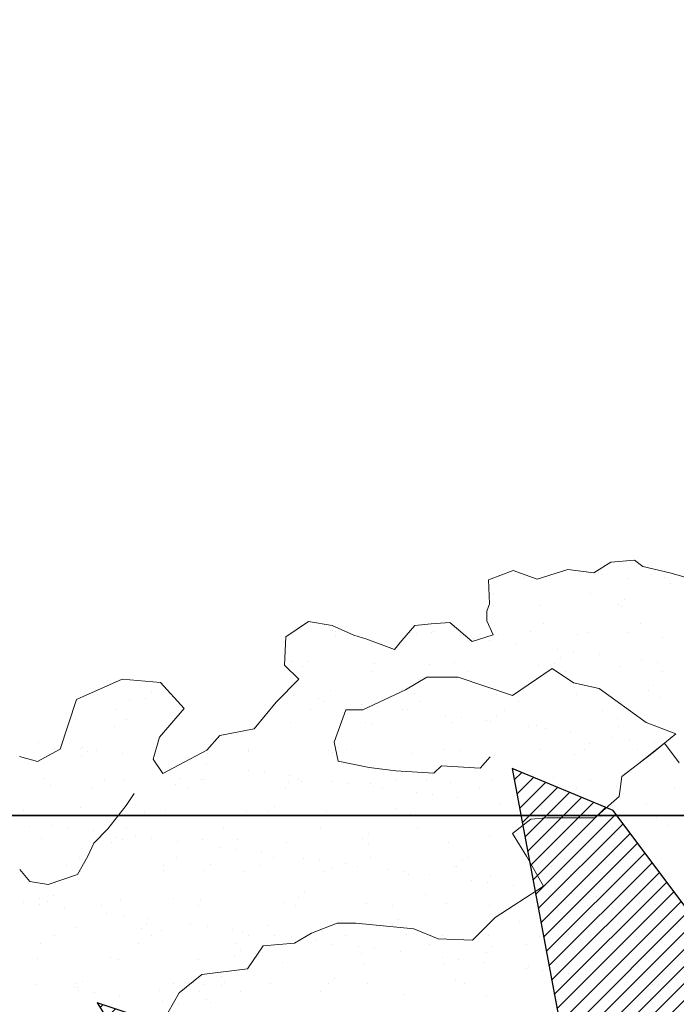
# Model space of a CAD drawing. Units: inches. Extents: x 1986 to 21484, y -1816 to 2016.
# Tile 36 of 85: x 2159.57 to 2167.98, y 1898.33 to 1910.95. Entities that reach past the tile are written whole.
import ezdxf

# ---------------------------------------------------------------- set-up
doc = ezdxf.new("R2010")
doc.units = ezdxf.units.IN
for name, color, linetype, lineweight in [('A-ANNO-DIMS', 2, 'Continuous', 18), ('C-PROP', 7, 'Continuous', 35), ('L-PLNT', 84, 'Continuous', 13), ('vfolhas', 114, 'Continuous', 5)]:
    doc.layers.add(name, color=color, linetype=linetype, lineweight=lineweight)
doc.layers.add('vfolha2', color=110, linetype='Continuous')
doc.layers.add('vfolhas2', color=102, linetype='Continuous')
doc.styles.get("Standard").update_dxf_attribs({"font": 'arial.ttf'})
doc.dimstyles.new('ISO-25', dxfattribs={"dimtxt": 8, "dimasz": 2.5, "dimexe": 1.25, "dimexo": 0.625, "dimtad": 1, "dimdec": 1, "dimlunit": 3, "dimtxsty": 'Standard', "dimcen": 2.5, "dimadec": 0, "dimazin": 0, "dimtfac": 1, "dimtdec": 1, "dimtmove": 0, "dimatfit": 3, "dimfxl": 1, "dimarcsym": 0})
pattern_1 = [(45, (-2446.5133113, 50.986076), (-0.004419417382, 0.004419417382), [])]

# ---------------------------------------------------------------- blocks, each defined once
blk = doc.blocks.new('*D1')
at = {"layer": 'A-ANNO-DIMS', "color": 0, "lineweight": -2, "transparency": 16777216}
for p, q in [((2042.312, 1901.377), (2042.312, 1914.655)), ((2402.312, 1901.377), (2402.312, 1914.655)), ((2044.812, 1913.405), (2399.812, 1913.405))]:
    blk.add_line(p, q, dxfattribs=at)
at = {"layer": 'A-ANNO-DIMS', "color": 0, "transparency": 16777216}
for points in [[(2044.812, 1913.821), (2044.812, 1912.988), (2042.312, 1913.405)], [(2399.812, 1913.821), (2399.812, 1912.988), (2402.312, 1913.405)]]:
    blk.add_solid(points, dxfattribs=at)
at = {"layer": 'Defpoints', "color": 0, "transparency": 16777216}
for p in [(2402.312, 1913.405), (2042.312, 1900.752), (2402.312, 1900.752)]:
    blk.add_point(p, dxfattribs=at)
at = {"layer": 'A-ANNO-DIMS', "color": 0, "transparency": 16777216, "insert": (2222.312, 1918.117), "char_height": 8, "attachment_point": 5}
blk.add_mtext("30'", dxfattribs=at)
blk = doc.blocks.new('arbusto_PB_verde_grande')
at = {"layer": 'vfolha2'}
h = blk.add_hatch(dxfattribs=at)
h.set_pattern_fill('ANSI31', color=256, scale=0.05, style=0)
h.set_pattern_definition(pattern_1)
h.paths.add_polyline_path([(-0.18963, 0.29704), (-0.08553, 0.20192), (-0.10785, 0.25007), (-0.13202, 0.31865), (-0.25096, 0.48479), (-0.44952, 0.5505), (-0.37946, 0.43789)])
h.paths.add_polyline_path([(0.07911, -0.4071), (0.08214, -0.50631), (0.17255, -0.6355), (0.18428, -0.44151), (0.14904, -0.29177), (0.02625, -0.03934), (0.03527, -0.25376)])
at = {"layer": 'vfolhas'}
h = blk.add_hatch(dxfattribs=at)
h.set_pattern_fill('ANSI31', color=256, scale=0.05, style=0)
h.set_pattern_definition(pattern_1)
h.paths.add_polyline_path([(-0.07279, 0.50669), (-0.18085, 0.65063), (-0.2334, 0.67253), (-0.20712, 0.53176), (-0.10785, 0.25007), (0.02625, -0.03934), (0.00028, 0.09048), (0.00816, 0.16241), (-0.04939, 0.29079)])
h.paths.add_polyline_path([(0.09902, 0.41929), (0.09372, 0.26573), (0.07906, 0.18814), (0.15506, 0.36901), (0.26606, 0.5505), (0.28356, 0.63504), (0.2485, 0.68819), (0.25145, 0.63504), (0.20178, 0.54426)])
h.paths.add_polyline_path([(0.12295, 0.24073), (0.047, 0.06233), (0.02625, -0.03934), (0.11122, 0.04358), (0.18428, 0.09364), (0.27478, 0.19376), (0.3215, 0.25323), (0.44129, 0.38467), (0.47634, 0.57866), (0.41789, 0.45347), (0.28939, 0.30954)])
h.paths.add_polyline_path([(0.58145, -0.03779), (0.70707, 0.01536), (0.78591, 0.04667), (0.74796, 0.06549), (0.62818, 0.08423), (0.52595, 0.09048), (0.39745, 0.04358), (0.02625, -0.03934), (0.25728, -0.03154), (0.43834, -0.0347)])
h.paths.add_polyline_path([(0.52022, -0.03647), (0.43834, -0.0347), (0.25728, -0.03154), (0.02625, -0.03934), (0.17964, -0.08515), (0.53768, -0.13167), (0.69541, -0.15357), (0.78591, -0.07852), (0.70413, -0.10042)])
h.paths.add_polyline_path([(0.27189, -0.21929), (0.14922, -0.14107), (0.02625, -0.03934), (0.15794, -0.31007), (0.29522, -0.42585), (0.41789, -0.49157), (0.56396, -0.56669), (0.5114, -0.48532), (0.39456, -0.34139)])
h.paths.add_polyline_path([(-0.05818, -0.47591), (-0.02312, -0.61984), (0.047, -0.80134), (0.08494, -0.59794), (0.07911, -0.4071), (0.03527, -0.25376), (0.02625, -0.03934), (-0.03773, -0.26001)])
h.paths.add_polyline_path([(-0.24218, 0.14054), (-0.11073, 0.06858), (0.02625, -0.03934), (-0.04235, 0.10871), (-0.21007, 0.23757), (-0.36485, 0.33145), (-0.47874, 0.40341), (-0.54303, 0.46288), (-0.49041, 0.33145), (-0.39408, 0.22192)])
at = {"layer": 'vfolha2'}
for p, q in [((-0.44952, 0.5505), (-0.37946, 0.43789)), ((-0.25096, 0.48479), (-0.44952, 0.5505))]:
    blk.add_line(p, q, dxfattribs=at)
at = {"layer": 'vfolhas2'}
for p, q in [((-0.2334, 0.67253), (-0.20712, 0.53176)), ((-0.18085, 0.65063), (-0.2334, 0.67253)), ((-0.07279, 0.50669), (-0.18085, 0.65063))]:
    blk.add_line(p, q, dxfattribs=at)
blk = doc.blocks.new('PLANT-SHRUB')
for p, q in [((2166.926, 1903.86), (2167.146, 1903.999)), ((2167.146, 1903.999), (2167.447, 1904.021)), ((2167.447, 1904.021), (2167.557, 1903.941)), ((2167.557, 1903.941), (2167.902, 1903.86)), ((2165.577, 1903.772), (2165.892, 1903.889)), ((2165.892, 1903.889), (2166.2, 1903.779)), ((2166.039, 1903.805), (2166.039, 1903.805)), ((2166.2, 1903.779), (2166.596, 1903.904)), ((2166.596, 1903.904), (2166.926, 1903.86)), ((2166.749, 1903.841), (2166.749, 1903.841)), ((2166.833, 1903.864), (2166.833, 1903.864)), ((2167.041, 1903.837), (2167.041, 1903.837)), ((2167.662, 1903.84), (2167.662, 1903.84)), ((2167.902, 1903.86), (2168.188, 1903.779)), ((2165.577, 1903.772), (2165.577, 1903.772)), ((2165.591, 1903.464), (2165.577, 1903.772)), ((2167.366, 1903.794), (2167.366, 1903.794)), ((2167.829, 1903.802), (2167.829, 1903.802)), ((2167.908, 1903.723), (2167.908, 1903.723)), ((2165.642, 1903.599), (2165.642, 1903.599)), ((2166.886, 1903.597), (2166.886, 1903.597)), ((2165.555, 1903.369), (2165.591, 1903.464)), ((2165.641, 1903.44), (2165.641, 1903.44)), ((2166.242, 1903.44), (2166.242, 1903.44)), ((2167.24, 1903.454), (2167.24, 1903.454)), ((2167.288, 1903.427), (2167.288, 1903.427)), ((2167.314, 1903.522), (2167.314, 1903.522)), ((2165.555, 1903.244), (2165.555, 1903.369)), ((2162.98, 1903.039), (2163.272, 1903.237)), ((2163.272, 1903.237), (2163.572, 1903.185)), ((2163.572, 1903.185), (2163.851, 1903.061)), ((2164.467, 1902.995), (2164.635, 1903.185)), ((2164.635, 1903.185), (2164.841, 1903.207)), ((2164.841, 1903.207), (2165.083, 1903.222)), ((2165.035, 1903.212), (2165.035, 1903.212)), ((2165.083, 1903.222), (2165.369, 1902.98)), ((2165.635, 1903.068), (2165.555, 1903.244)), ((2166.28, 1903.21), (2166.28, 1903.21)), ((2167.524, 1903.208), (2167.524, 1903.208)), ((2163.576, 1903.118), (2163.576, 1903.118)), ((2163.622, 1903.107), (2163.622, 1903.107)), ((2163.851, 1903.061), (2164.019, 1903.009)), ((2164.655, 1903.079), (2164.655, 1903.079)), ((2164.845, 1903.091), (2164.845, 1903.091)), ((2164.866, 1903.105), (2164.866, 1903.105)), ((2165.22, 1903.054), (2165.22, 1903.054)), ((2165.369, 1902.98), (2165.635, 1903.068)), ((2165.702, 1903.066), (2165.702, 1903.066)), ((2166.111, 1903.103), (2166.111, 1903.103)), ((2166.724, 1903.071), (2166.724, 1903.071)), ((2166.842, 1903.09), (2166.842, 1903.09)), ((2167.356, 1903.1), (2167.356, 1903.1)), ((2162.964, 1902.679), (2162.98, 1903.039)), ((2163.62, 1903.041), (2163.62, 1903.041)), ((2164.019, 1903.009), (2164.371, 1902.878)), ((2164.371, 1902.878), (2164.467, 1902.995)), ((2165.369, 1902.98), (2165.369, 1902.98)), ((2165.369, 1902.98), (2165.369, 1902.98)), ((2165.388, 1903.02), (2165.388, 1903.02)), ((2165.596, 1902.992), (2165.596, 1902.992)), ((2165.921, 1902.949), (2165.921, 1902.949)), ((2167.803, 1903.032), (2167.803, 1903.032)), ((2166.464, 1902.878), (2166.464, 1902.878)), ((2166.672, 1902.851), (2166.672, 1902.851)), ((2166.997, 1902.808), (2166.997, 1902.808)), ((2163.147, 1902.496), (2162.964, 1902.679)), ((2163.069, 1902.718), (2163.069, 1902.718)), ((2163.273, 1902.722), (2163.273, 1902.722)), ((2164.115, 1902.704), (2164.115, 1902.704)), ((2164.822, 1902.69), (2164.822, 1902.69)), ((2165.137, 1902.709), (2165.137, 1902.709)), ((2166.217, 1902.67), (2166.217, 1902.67)), ((2166.421, 1902.704), (2166.421, 1902.704)), ((2166.495, 1902.771), (2166.495, 1902.771)), ((2167.54, 1902.736), (2167.54, 1902.736)), ((2167.748, 1902.709), (2167.748, 1902.709)), ((2163.199, 1902.654), (2163.199, 1902.654)), ((2164.074, 1902.6), (2164.074, 1902.6)), ((2165.319, 1902.598), (2165.319, 1902.598)), ((2166.393, 1902.634), (2165.883, 1902.288)), ((2166.393, 1902.634), (2166.393, 1902.634)), ((2166.667, 1902.452), (2166.393, 1902.634)), ((2166.564, 1902.596), (2166.564, 1902.596)), ((2167.263, 1902.657), (2167.263, 1902.657)), ((2167.808, 1902.594), (2167.808, 1902.594)), ((2160.298, 1902.236), (2160.882, 1902.496)), ((2160.882, 1902.496), (2161.373, 1902.455)), ((2161.373, 1902.455), (2161.676, 1902.121)), ((2162.855, 1902.204), (2163.147, 1902.496)), ((2164.788, 1902.524), (2164.515, 1902.36)), ((2164.788, 1902.524), (2164.788, 1902.524)), ((2165.19, 1902.524), (2164.788, 1902.524)), ((2165.883, 1902.288), (2165.19, 1902.524)), ((2166.667, 1902.452), (2166.667, 1902.452)), ((2166.995, 1902.379), (2166.667, 1902.452)), ((2167.696, 1902.42), (2167.696, 1902.42)), ((2161.252, 1902.322), (2161.252, 1902.322)), ((2163.551, 1902.348), (2163.551, 1902.348)), ((2164.515, 1902.36), (2163.967, 1902.105)), ((2164.4, 1902.304), (2164.4, 1902.304)), ((2164.474, 1902.371), (2164.474, 1902.371)), ((2164.63, 1902.309), (2164.63, 1902.309)), ((2165.676, 1902.296), (2165.676, 1902.296)), ((2166.023, 1902.339), (2166.023, 1902.339)), ((2166.699, 1902.3), (2166.699, 1902.3)), ((2167.597, 1901.941), (2166.995, 1902.379)), ((2167.622, 1902.353), (2167.622, 1902.353)), ((2160.089, 1901.6), (2160.298, 1902.236)), ((2160.978, 1902.218), (2160.978, 1902.218)), ((2161.178, 1902.255), (2161.178, 1902.255)), ((2162.573, 1901.86), (2162.855, 1902.204)), ((2163.076, 1902.289), (2163.076, 1902.289)), ((2163.401, 1902.246), (2163.401, 1902.246)), ((2163.468, 1902.214), (2163.468, 1902.214)), ((2163.944, 1902.175), (2163.944, 1902.175)), ((2164.712, 1902.212), (2164.712, 1902.212)), ((2165.957, 1902.209), (2165.957, 1902.209)), ((2167.201, 1902.207), (2167.201, 1902.207)), ((2167.778, 1902.262), (2167.778, 1902.262)), ((2160.81, 1902.111), (2160.81, 1902.111)), ((2161.676, 1902.121), (2161.362, 1901.756)), ((2163.299, 1902.106), (2163.299, 1902.106)), ((2163.75, 1902.105), (2163.597, 1901.691)), ((2163.967, 1902.105), (2163.75, 1902.105)), ((2164.152, 1902.148), (2164.152, 1902.148)), ((2164.477, 1902.105), (2164.477, 1902.105)), ((2164.544, 1902.104), (2164.544, 1902.104)), ((2165.788, 1902.102), (2165.788, 1902.102)), ((2167.033, 1902.1), (2167.033, 1902.1)), ((2160.942, 1901.982), (2160.942, 1901.982)), ((2163.044, 1901.948), (2163.044, 1901.948)), ((2164.003, 1901.939), (2164.003, 1901.939)), ((2164.09, 1901.934), (2164.09, 1901.934)), ((2165.02, 1902.033), (2165.02, 1902.033)), ((2165.112, 1901.939), (2165.112, 1901.939)), ((2165.228, 1902.006), (2165.228, 1902.006)), ((2165.553, 1901.963), (2165.553, 1901.963)), ((2165.602, 1901.953), (2165.602, 1901.953)), ((2165.675, 1902.02), (2165.675, 1902.02)), ((2167.225, 1901.988), (2167.225, 1901.988)), ((2167.597, 1901.941), (2167.597, 1901.941)), ((2167.979, 1901.796), (2167.597, 1901.941)), ((2160.78, 1901.89), (2160.78, 1901.89)), ((2162.135, 1901.777), (2162.573, 1901.86)), ((2162.573, 1901.86), (2162.573, 1901.86)), ((2166.096, 1901.892), (2166.096, 1901.892)), ((2166.192, 1901.9), (2166.192, 1901.9)), ((2166.304, 1901.864), (2166.304, 1901.864)), ((2166.629, 1901.821), (2166.629, 1901.821)), ((2167.238, 1901.887), (2167.238, 1901.887)), ((2167.688, 1901.559), (2167.979, 1901.796)), ((2159.805, 1901.685), (2159.805, 1901.685)), ((2161.362, 1901.756), (2161.279, 1901.474)), ((2161.968, 1901.589), (2162.135, 1901.777)), ((2163.597, 1901.691), (2163.651, 1901.448)), ((2163.597, 1901.691), (2163.597, 1901.691)), ((2166.877, 1901.67), (2166.877, 1901.67)), ((2167.171, 1901.75), (2167.171, 1901.75)), ((2167.379, 1901.723), (2167.379, 1901.723)), ((2167.487, 1901.404), (2167.834, 1901.677)), ((2167.704, 1901.68), (2167.704, 1901.68)), ((2167.834, 1901.677), (2168.02, 1901.424)), ((2159.797, 1901.443), (2160.089, 1901.6)), ((2160.018, 1901.606), (2160.018, 1901.606)), ((2160.348, 1901.614), (2160.348, 1901.614)), ((2160.377, 1901.625), (2160.377, 1901.625)), ((2160.433, 1901.571), (2160.433, 1901.571)), ((2160.556, 1901.586), (2160.556, 1901.586)), ((2160.881, 1901.543), (2160.881, 1901.543)), ((2161.404, 1901.287), (2161.968, 1901.589)), ((2161.982, 1901.539), (2161.982, 1901.539)), ((2162.503, 1901.573), (2162.503, 1901.573)), ((2162.507, 1901.602), (2162.507, 1901.602)), ((2163.526, 1901.578), (2163.526, 1901.578)), ((2163.581, 1901.553), (2163.581, 1901.553)), ((2163.655, 1901.621), (2163.655, 1901.621)), ((2163.751, 1901.6), (2163.751, 1901.6)), ((2164.605, 1901.539), (2164.605, 1901.539)), ((2164.996, 1901.597), (2164.996, 1901.597)), ((2165.204, 1901.588), (2165.204, 1901.588)), ((2166.241, 1901.595), (2166.241, 1901.595)), ((2166.803, 1901.602), (2166.803, 1901.602)), ((2167.287, 1901.249), (2167.688, 1901.559)), ((2167.485, 1901.593), (2167.485, 1901.593)), ((2167.688, 1901.559), (2167.688, 1901.559)), ((2159.568, 1901.506), (2159.797, 1901.443)), ((2160.359, 1901.504), (2160.359, 1901.504)), ((2161.279, 1901.474), (2161.404, 1901.287)), ((2163.651, 1901.448), (2164.048, 1901.367)), ((2163.651, 1901.448), (2163.651, 1901.448)), ((2165.471, 1901.358), (2165.597, 1901.502)), ((2165.597, 1901.502), (2165.597, 1901.502)), ((2165.651, 1901.525), (2165.651, 1901.525)), ((2166.674, 1901.53), (2166.674, 1901.53)), ((2167.753, 1901.492), (2167.753, 1901.492)), ((2161.957, 1901.402), (2161.957, 1901.402)), ((2162.5, 1901.33), (2162.5, 1901.33)), ((2162.708, 1901.303), (2162.708, 1901.303)), ((2164.048, 1901.367), (2164.39, 1901.322)), ((2164.39, 1901.322), (2164.876, 1901.295)), ((2164.876, 1901.295), (2164.975, 1901.385)), ((2164.975, 1901.385), (2165.471, 1901.358)), ((2165.471, 1901.358), (2165.471, 1901.358)), ((2159.87, 1901.225), (2159.87, 1901.225)), ((2160.655, 1901.218), (2160.655, 1901.218)), ((2160.917, 1901.211), (2160.917, 1901.211)), ((2161.634, 1901.221), (2161.634, 1901.221)), ((2161.9, 1901.215), (2161.9, 1901.215)), ((2161.939, 1901.216), (2161.939, 1901.216)), ((2163.018, 1901.177), (2163.018, 1901.177)), ((2163.033, 1901.26), (2163.033, 1901.26)), ((2163.145, 1901.213), (2163.145, 1901.213)), ((2163.183, 1901.189), (2163.183, 1901.189)), ((2163.575, 1901.189), (2163.575, 1901.189)), ((2163.783, 1901.161), (2163.783, 1901.161)), ((2164.065, 1901.164), (2164.065, 1901.164)), ((2164.389, 1901.211), (2164.389, 1901.211)), ((2164.783, 1901.202), (2164.783, 1901.202)), ((2164.856, 1901.27), (2164.856, 1901.27)), ((2165.087, 1901.169), (2165.087, 1901.169)), ((2165.634, 1901.208), (2165.634, 1901.208)), ((2166.405, 1901.238), (2166.405, 1901.238)), ((2166.879, 1901.206), (2166.879, 1901.206)), ((2167.25, 1900.994), (2167.287, 1901.249)), ((2159.961, 1901.139), (2159.961, 1901.139)), ((2160.487, 1901.11), (2160.487, 1901.11)), ((2160.933, 1900.878), (2161.037, 1901.034)), ((2161.561, 1901.153), (2161.561, 1901.153)), ((2161.732, 1901.108), (2161.732, 1901.108)), ((2162.976, 1901.106), (2162.976, 1901.106)), ((2164.108, 1901.118), (2164.108, 1901.118)), ((2164.221, 1901.103), (2164.221, 1901.103)), ((2164.651, 1901.047), (2164.651, 1901.047)), ((2165.465, 1901.101), (2165.465, 1901.101)), ((2166.166, 1901.13), (2166.166, 1901.13)), ((2166.71, 1901.099), (2166.71, 1901.099)), ((2167.213, 1901.117), (2167.213, 1901.117)), ((2167.955, 1901.097), (2167.955, 1901.097)), ((2164.859, 1901.02), (2164.859, 1901.02)), ((2165.184, 1900.977), (2165.184, 1900.977)), ((2165.727, 1900.905), (2165.727, 1900.905)), ((2166.058, 1900.919), (2166.058, 1900.919)), ((2166.94, 1900.721), (2167.25, 1900.994)), ((2167.25, 1900.994), (2167.25, 1900.994)), ((2167.25, 1900.994), (2167.25, 1900.994)), ((2159.614, 1900.821), (2159.614, 1900.821)), ((2160.352, 1900.855), (2160.352, 1900.855)), ((2160.7, 1900.579), (2160.933, 1900.878)), ((2161.163, 1900.789), (2161.163, 1900.789)), ((2161.432, 1900.816), (2161.432, 1900.816)), ((2162.478, 1900.803), (2162.478, 1900.803)), ((2162.762, 1900.802), (2162.762, 1900.802)), ((2162.836, 1900.87), (2162.836, 1900.87)), ((2163.5, 1900.808), (2163.5, 1900.808)), ((2164.385, 1900.838), (2164.385, 1900.838)), ((2165.935, 1900.878), (2165.935, 1900.878)), ((2165.984, 1900.851), (2165.984, 1900.851)), ((2166.26, 1900.835), (2166.26, 1900.835)), ((2167.607, 1900.887), (2167.607, 1900.887)), ((2164.58, 1900.769), (2164.58, 1900.769)), ((2165.626, 1900.755), (2165.626, 1900.755)), ((2165.883, 1900.52), (2166.12, 1900.702)), ((2166.12, 1900.702), (2166.32, 1900.721)), ((2166.32, 1900.721), (2166.612, 1900.721)), ((2166.612, 1900.721), (2166.94, 1900.721)), ((2166.648, 1900.76), (2166.648, 1900.76)), ((2166.803, 1900.764), (2166.803, 1900.764)), ((2166.94, 1900.721), (2166.94, 1900.721)), ((2167.011, 1900.736), (2167.011, 1900.736)), ((2167.336, 1900.694), (2167.336, 1900.694)), ((2167.728, 1900.721), (2167.728, 1900.721)), ((2159.695, 1900.606), (2159.695, 1900.606)), ((2159.979, 1900.627), (2159.979, 1900.627)), ((2160.188, 1900.6), (2160.188, 1900.6)), ((2160.512, 1900.557), (2160.512, 1900.557)), ((2160.518, 1900.398), (2160.7, 1900.579)), ((2160.7, 1900.579), (2160.7, 1900.579)), ((2160.939, 1900.603), (2160.939, 1900.603)), ((2162.184, 1900.601), (2162.184, 1900.601)), ((2163.429, 1900.599), (2163.429, 1900.599)), ((2164.673, 1900.596), (2164.673, 1900.596)), ((2165.918, 1900.594), (2165.918, 1900.594)), ((2167.163, 1900.592), (2167.163, 1900.592)), ((2167.259, 1900.568), (2167.259, 1900.568)), ((2167.879, 1900.622), (2167.879, 1900.622)), ((2159.845, 1900.455), (2159.845, 1900.455)), ((2160.44, 1900.229), (2160.518, 1900.398)), ((2160.741, 1900.403), (2160.741, 1900.403)), ((2160.815, 1900.47), (2160.815, 1900.47)), ((2160.891, 1900.441), (2160.891, 1900.441)), ((2161.055, 1900.486), (2161.055, 1900.486)), ((2161.263, 1900.458), (2161.263, 1900.458)), ((2161.588, 1900.415), (2161.588, 1900.415)), ((2161.914, 1900.446), (2161.914, 1900.446)), ((2162.364, 1900.438), (2162.364, 1900.438)), ((2162.993, 1900.407), (2162.993, 1900.407)), ((2163.963, 1900.452), (2163.963, 1900.452)), ((2164.037, 1900.519), (2164.037, 1900.519)), ((2165.062, 1900.399), (2165.062, 1900.399)), ((2165.586, 1900.487), (2165.586, 1900.487)), ((2166.065, 1900.229), (2165.883, 1900.52)), ((2167.186, 1900.501), (2167.186, 1900.501)), ((2162.131, 1900.344), (2162.131, 1900.344)), ((2162.339, 1900.317), (2162.339, 1900.317)), ((2162.664, 1900.274), (2162.664, 1900.274)), ((2164.039, 1900.394), (2164.039, 1900.394)), ((2166.141, 1900.36), (2166.141, 1900.36)), ((2167.187, 1900.347), (2167.187, 1900.347)), ((2160.31, 1899.995), (2160.44, 1900.229)), ((2160.333, 1900.217), (2160.333, 1900.217)), ((2161.577, 1900.214), (2161.577, 1900.214)), ((2162.822, 1900.212), (2162.822, 1900.212)), ((2163.207, 1900.202), (2163.207, 1900.202)), ((2163.415, 1900.175), (2163.415, 1900.175)), ((2164.067, 1900.21), (2164.067, 1900.21)), ((2165.239, 1900.168), (2165.239, 1900.168)), ((2165.311, 1900.208), (2165.311, 1900.208)), ((2166.065, 1900.229), (2166.065, 1900.229)), ((2166.284, 1899.846), (2166.065, 1900.229)), ((2166.556, 1900.205), (2166.556, 1900.205)), ((2167.8, 1900.203), (2167.8, 1900.203)), ((2159.569, 1900.06), (2159.699, 1899.904)), ((2160.164, 1900.109), (2160.164, 1900.109)), ((2160.327, 1900.085), (2160.327, 1900.085)), ((2160.344, 1900.038), (2160.344, 1900.038)), ((2161.407, 1900.046), (2161.407, 1900.046)), ((2161.409, 1900.107), (2161.409, 1900.107)), ((2161.943, 1900.052), (2161.943, 1900.052)), ((2162.016, 1900.119), (2162.016, 1900.119)), ((2162.453, 1900.033), (2162.453, 1900.033)), ((2162.653, 1900.105), (2162.653, 1900.105)), ((2163.475, 1900.038), (2163.475, 1900.038)), ((2163.566, 1900.087), (2163.566, 1900.087)), ((2163.74, 1900.132), (2163.74, 1900.132)), ((2163.898, 1900.103), (2163.898, 1900.103)), ((2164.283, 1900.061), (2164.283, 1900.061)), ((2164.491, 1900.033), (2164.491, 1900.033)), ((2165.143, 1900.1), (2165.143, 1900.1)), ((2165.165, 1900.101), (2165.165, 1900.101)), ((2166.387, 1900.098), (2166.387, 1900.098)), ((2166.788, 1900.136), (2166.788, 1900.136)), ((2167.632, 1900.096), (2167.632, 1900.096)), ((2159.699, 1899.904), (2159.933, 1899.865)), ((2159.933, 1899.865), (2160.31, 1899.995)), ((2164.555, 1899.999), (2164.555, 1899.999)), ((2164.816, 1899.991), (2164.816, 1899.991)), ((2165.359, 1899.919), (2165.359, 1899.919)), ((2165.601, 1899.985), (2165.601, 1899.985)), ((2166.623, 1899.99), (2166.623, 1899.99)), ((2167.703, 1899.951), (2167.703, 1899.951)), ((2163.218, 1899.768), (2163.218, 1899.768)), ((2165.567, 1899.892), (2165.567, 1899.892)), ((2165.662, 1899.443), (2166.284, 1899.846)), ((2165.892, 1899.849), (2165.892, 1899.849)), ((2166.434, 1899.777), (2166.434, 1899.777)), ((2166.44, 1899.818), (2166.44, 1899.818)), ((2159.611, 1899.641), (2159.611, 1899.641)), ((2159.82, 1899.685), (2159.82, 1899.685)), ((2159.922, 1899.652), (2159.922, 1899.652)), ((2159.996, 1899.719), (2159.996, 1899.719)), ((2160.866, 1899.671), (2160.866, 1899.671)), ((2161.545, 1899.687), (2161.545, 1899.687)), ((2161.889, 1899.676), (2161.889, 1899.676)), ((2163.144, 1899.701), (2163.144, 1899.701)), ((2164.767, 1899.736), (2164.767, 1899.736)), ((2166.366, 1899.75), (2166.366, 1899.75)), ((2166.642, 1899.75), (2166.642, 1899.75)), ((2166.967, 1899.707), (2166.967, 1899.707)), ((2159.819, 1899.614), (2159.819, 1899.614)), ((2160.144, 1899.571), (2160.144, 1899.571)), ((2160.617, 1899.602), (2160.617, 1899.602)), ((2161.861, 1899.6), (2161.861, 1899.6)), ((2162.968, 1899.637), (2162.968, 1899.637)), ((2163.106, 1899.598), (2163.106, 1899.598)), ((2164.014, 1899.624), (2164.014, 1899.624)), ((2164.351, 1899.596), (2164.351, 1899.596)), ((2165.037, 1899.629), (2165.037, 1899.629)), ((2165.595, 1899.593), (2165.595, 1899.593)), ((2166.116, 1899.59), (2166.116, 1899.59)), ((2166.84, 1899.591), (2166.84, 1899.591)), ((2167.162, 1899.577), (2167.162, 1899.577)), ((2167.51, 1899.636), (2167.51, 1899.636)), ((2167.718, 1899.608), (2167.718, 1899.608)), ((2160.687, 1899.499), (2160.687, 1899.499)), ((2160.895, 1899.472), (2160.895, 1899.472)), ((2161.22, 1899.429), (2161.22, 1899.429)), ((2164.419, 1899.418), (2164.419, 1899.418)), ((2165.37, 1899.152), (2165.662, 1899.443)), ((2167.568, 1899.399), (2167.568, 1899.399)), ((2167.641, 1899.467), (2167.641, 1899.467)), ((2160.302, 1899.315), (2160.302, 1899.315)), ((2161.124, 1899.301), (2161.124, 1899.301)), ((2161.197, 1899.369), (2161.197, 1899.369)), ((2161.381, 1899.276), (2161.381, 1899.276)), ((2161.763, 1899.358), (2161.763, 1899.358)), ((2161.971, 1899.33), (2161.971, 1899.33)), ((2162.296, 1899.287), (2162.296, 1899.287)), ((2162.428, 1899.263), (2162.428, 1899.263)), ((2162.746, 1899.336), (2162.746, 1899.336)), ((2163.309, 1899.243), (2163.638, 1899.37)), ((2163.45, 1899.267), (2163.45, 1899.267)), ((2163.638, 1899.37), (2163.875, 1899.37)), ((2163.875, 1899.37), (2164.622, 1899.297)), ((2164.346, 1899.35), (2164.346, 1899.35)), ((2164.622, 1899.297), (2164.932, 1899.17)), ((2165.969, 1899.386), (2165.969, 1899.386)), ((2160.01, 1899.216), (2160.01, 1899.216)), ((2161.255, 1899.214), (2161.255, 1899.214)), ((2162.499, 1899.211), (2162.499, 1899.211)), ((2162.838, 1899.216), (2162.838, 1899.216)), ((2163.046, 1899.189), (2163.046, 1899.189)), ((2163.091, 1899.115), (2163.309, 1899.243)), ((2163.371, 1899.146), (2163.371, 1899.146)), ((2163.744, 1899.209), (2163.744, 1899.209)), ((2164.529, 1899.229), (2164.529, 1899.229)), ((2164.932, 1899.17), (2165.37, 1899.152)), ((2164.988, 1899.207), (2164.988, 1899.207)), ((2165.37, 1899.152), (2165.37, 1899.152)), ((2165.576, 1899.215), (2165.576, 1899.215)), ((2166.233, 1899.205), (2166.233, 1899.205)), ((2166.598, 1899.22), (2166.598, 1899.22)), ((2167.478, 1899.202), (2167.478, 1899.202)), ((2167.677, 1899.181), (2167.677, 1899.181)), ((2159.841, 1899.109), (2159.841, 1899.109)), ((2161.086, 1899.106), (2161.086, 1899.106)), ((2162.331, 1899.104), (2162.331, 1899.104)), ((2162.399, 1899.018), (2162.399, 1899.018)), ((2162.489, 1898.787), (2162.689, 1899.079)), ((2162.689, 1899.079), (2163.091, 1899.115)), ((2163.575, 1899.102), (2163.575, 1899.102)), ((2163.914, 1899.074), (2163.914, 1899.074)), ((2164.122, 1899.047), (2164.122, 1899.047)), ((2164.82, 1899.099), (2164.82, 1899.099)), ((2165.621, 1899.067), (2165.621, 1899.067)), ((2166.065, 1899.097), (2166.065, 1899.097)), ((2167.17, 1899.035), (2167.17, 1899.035)), ((2167.309, 1899.095), (2167.309, 1899.095)), ((2159.795, 1898.915), (2159.795, 1898.915)), ((2160.726, 1898.937), (2160.726, 1898.937)), ((2160.841, 1898.901), (2160.841, 1898.901)), ((2161.863, 1898.906), (2161.863, 1898.906)), ((2162.325, 1898.95), (2162.325, 1898.95)), ((2163.948, 1898.986), (2163.948, 1898.986)), ((2164.447, 1899.004), (2164.447, 1899.004)), ((2164.99, 1898.933), (2164.99, 1898.933)), ((2165.198, 1898.905), (2165.198, 1898.905)), ((2165.547, 1898.999), (2165.547, 1898.999)), ((2161.905, 1898.714), (2162.489, 1898.787)), ((2162.489, 1898.787), (2162.489, 1898.787)), ((2162.943, 1898.867), (2162.943, 1898.867)), ((2163.989, 1898.854), (2163.989, 1898.854)), ((2165.011, 1898.859), (2165.011, 1898.859)), ((2165.523, 1898.863), (2165.523, 1898.863)), ((2166.066, 1898.791), (2166.066, 1898.791)), ((2166.091, 1898.82), (2166.091, 1898.82)), ((2166.274, 1898.764), (2166.274, 1898.764)), ((2167.137, 1898.806), (2167.137, 1898.806)), ((2161.614, 1898.477), (2161.905, 1898.714)), ((2161.877, 1898.658), (2161.877, 1898.658)), ((2162.15, 1898.686), (2162.15, 1898.686)), ((2163.6, 1898.667), (2163.6, 1898.667)), ((2165.149, 1898.635), (2165.149, 1898.635)), ((2166.599, 1898.721), (2166.599, 1898.721)), ((2166.749, 1898.649), (2166.749, 1898.649)), ((2166.822, 1898.716), (2166.822, 1898.716)), ((2167.142, 1898.649), (2167.142, 1898.649)), ((2159.775, 1898.584), (2159.775, 1898.584)), ((2160.277, 1898.545), (2160.277, 1898.545)), ((2160.294, 1898.602), (2160.294, 1898.602)), ((2160.304, 1898.55), (2160.304, 1898.55)), ((2160.318, 1898.513), (2160.318, 1898.513)), ((2160.378, 1898.618), (2160.378, 1898.618)), ((2161.356, 1898.506), (2161.356, 1898.506)), ((2161.538, 1898.599), (2161.538, 1898.599)), ((2161.793, 1898.605), (2161.793, 1898.605)), ((2161.927, 1898.586), (2161.927, 1898.586)), ((2161.927, 1898.586), (2161.927, 1898.586)), ((2162.161, 1898.575), (2162.161, 1898.575)), ((2162.198, 1898.609), (2162.198, 1898.609)), ((2162.783, 1898.597), (2162.783, 1898.597)), ((2163.527, 1898.6), (2163.527, 1898.6)), ((2164.028, 1898.595), (2164.028, 1898.595)), ((2165.272, 1898.593), (2165.272, 1898.593)), ((2166.517, 1898.59), (2166.517, 1898.59)), ((2167.35, 1898.622), (2167.35, 1898.622)), ((2167.675, 1898.579), (2167.675, 1898.579)), ((2167.762, 1898.588), (2167.762, 1898.588)), ((2160.526, 1898.486), (2160.526, 1898.486)), ((2160.851, 1898.443), (2160.851, 1898.443)), ((2161.468, 1898.222), (2161.614, 1898.477)), ((2161.614, 1898.477), (2161.614, 1898.477)), ((2161.879, 1898.499), (2161.879, 1898.499)), ((2161.962, 1898.393), (2161.962, 1898.393)), ((2162.402, 1898.492), (2162.402, 1898.492)), ((2163.425, 1898.497), (2163.425, 1898.497)), ((2164.504, 1898.458), (2164.504, 1898.458)), ((2165.55, 1898.445), (2165.55, 1898.445)), ((2166.573, 1898.45), (2166.573, 1898.45)), ((2167.652, 1898.411), (2167.652, 1898.411)), ((2161.394, 1898.371), (2161.394, 1898.371)), ((2161.602, 1898.344), (2161.602, 1898.344)), ((2161.602, 1898.344), (2161.602, 1898.344)), ((2161.602, 1898.344), (2161.602, 1898.344)), ((2162.019, 1898.351), (2162.019, 1898.351))]:
    blk.add_line(p, q)

msp = doc.modelspace()

# ---------------------------------------------------------------- linework, layer by layer
at = {"layer": 'C-PROP'}
msp.add_lwpolyline([(2042.312, 1900.752), (2402.312, 1900.752), (2402.312, 1066.752), (2042.312, 1066.752)], close=True, dxfattribs=at)

# ---------------------------------------------------------------- block references
at = {"layer": 'L-PLNT'}
msp.add_blockref('PLANT-SHRUB', (0, 0), dxfattribs=at)
at = {"layer": 'L-PLNT', "xscale": 24.60366729364114, "yscale": 24.60366729364114, "zscale": 24.60366729364114}
msp.add_blockref('arbusto_PB_verde_grande', (2171.623, 1884.805), dxfattribs=at)

# ---------------------------------------------------------------- dimensions: what is measured, and where the dimension line sits
at = {"layer": 'A-ANNO-DIMS'}
dim = msp.add_linear_dim(base=(2402.312, 1913.405), p1=(2042.312, 1900.752), p2=(2402.312, 1900.752), dimstyle='ISO-25', override={"dimclrd": 0, "dimclre": 0, "dimclrt": 0}, dxfattribs=at)
dim.commit()
dim.dimension.update_dxf_attribs({"geometry": '*D1', "text_midpoint": (2222.312, 1918.117)})

doc.saveas('drawing.dxf')
